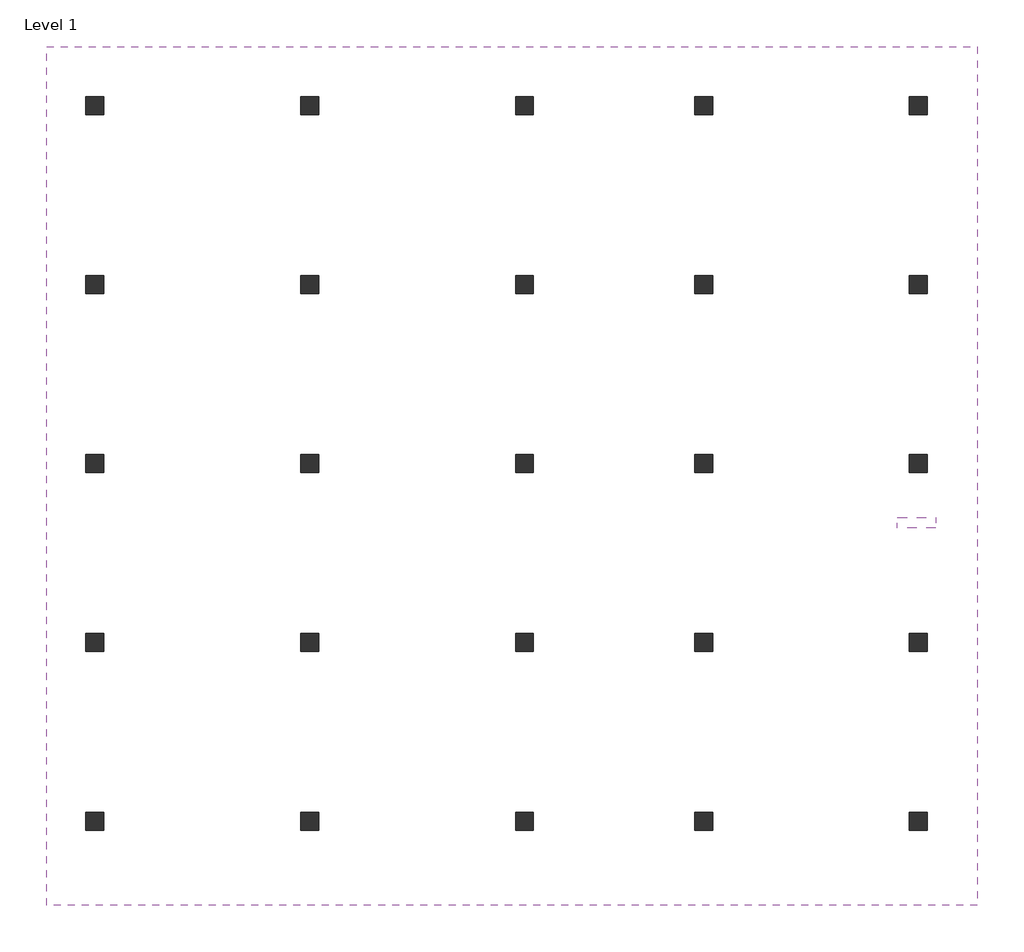
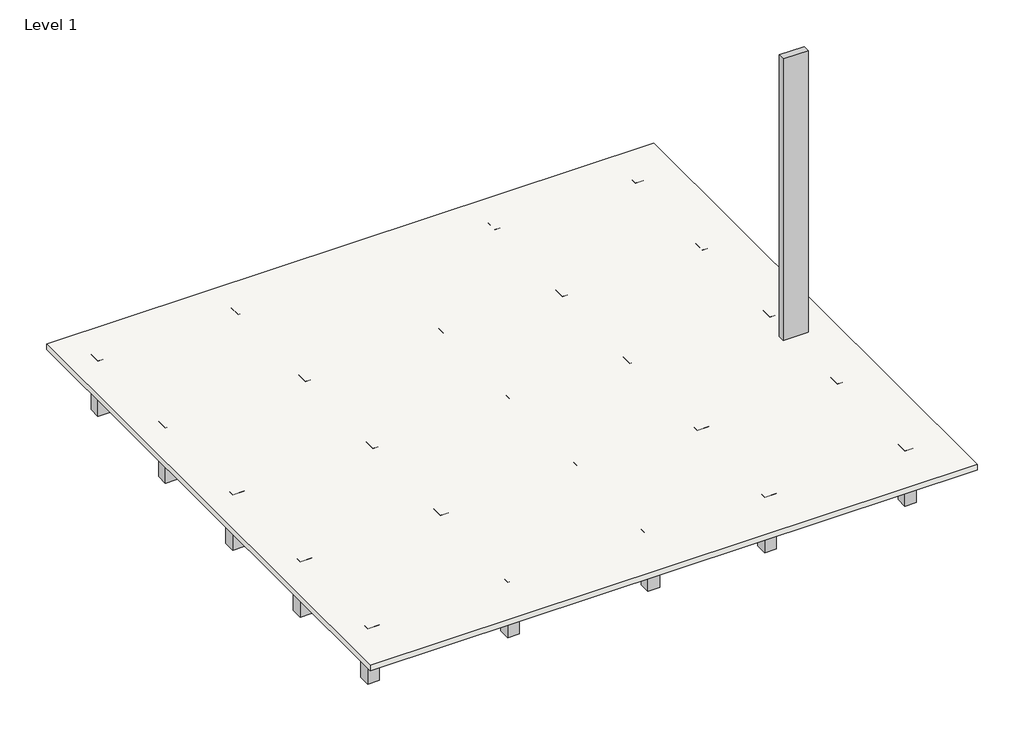
# One storey: 25 columns, 1 proxy, 1 slab.
"""IFC4 building model written with IfcOpenShell, lengths in millimetres."""

from ifc_helpers import new_model, si_unit, frame, origin, place, context, project, spatial, polyline, outline, extrude, transform, mapped, element, save
from components import generic_models_3_generic_models_3_f60183ce, column_c091e905

model = new_model("IFC4")

# Units and contexts
model_context = context("Model", 3, world=origin())
ifc_project = project(units=[si_unit("LENGTHUNIT", "METRE", prefix="MILLI")], contexts=[model_context])

# Site, building, storey
site = spatial("IfcSite", under=ifc_project)
building = spatial("IfcBuilding", under=site)
storey = spatial("IfcBuildingStorey", under=building, Name="Level 1", Elevation=0.0)

# Proxy
placement = place(None, origin())
generic_models_3_generic_models_3_shape = generic_models_3_generic_models_3_f60183ce(model_context)
element("IfcBuildingElementProxy", 1, Name="Generic Models 3 : Generic Models 3", ObjectType="Generic Models 3 : Generic Models 3", at=placement, inside=storey, context=model_context, shape_type="MappedRepresentation", body=[
    mapped(generic_models_3_generic_models_3_shape, transform((0.0, 0.0, 0.0), x_axis=(1.0, 0.0, 0.0), y_axis=(0.0, 1.0, 0.0), z_axis=(0.0, 0.0, 1.0))),
])

# Columns
column_shape = column_c091e905(model_context)
element("IfcColumn", 2, ObjectType="Rectangular Column : 24\" x 24\"", at=placement, inside=storey, context=model_context, shape_type="MappedRepresentation", body=[
    mapped(column_shape, transform((-13731.8638778, 14362.2237525, 0.0), x_axis=(1.0, 0.0, 0.0), y_axis=(0.0, 1.0, 0.0), z_axis=(0.0, 0.0, 1.0))),
])
element("IfcColumn", 3, ObjectType="Rectangular Column : 24\" x 24\"", at=placement, inside=storey, context=model_context, shape_type="MappedRepresentation", body=[
    mapped(column_shape, transform((-6416.6638778, 14362.2237525, 0.0), x_axis=(1.0, 0.0, 0.0), y_axis=(0.0, 1.0, 0.0), z_axis=(0.0, 0.0, 1.0))),
])
element("IfcColumn", 4, ObjectType="Rectangular Column : 24\" x 24\"", at=placement, inside=storey, context=model_context, shape_type="MappedRepresentation", body=[
    mapped(column_shape, transform((898.5361222, 14362.2237525, 0.0), x_axis=(1.0, 0.0, 0.0), y_axis=(0.0, 1.0, 0.0), z_axis=(0.0, 0.0, 1.0))),
])
element("IfcColumn", 5, ObjectType="Rectangular Column : 24\" x 24\"", at=placement, inside=storey, context=model_context, shape_type="MappedRepresentation", body=[
    mapped(column_shape, transform((6994.5361222, 14362.2237525, 0.0), x_axis=(1.0, 0.0, 0.0), y_axis=(0.0, 1.0, 0.0), z_axis=(0.0, 0.0, 1.0))),
])
element("IfcColumn", 6, ObjectType="Rectangular Column : 24\" x 24\"", at=placement, inside=storey, context=model_context, shape_type="MappedRepresentation", body=[
    mapped(column_shape, transform((14309.7361222, 14362.2237525, 0.0), x_axis=(1.0, 0.0, 0.0), y_axis=(0.0, 1.0, 0.0), z_axis=(0.0, 0.0, 1.0))),
])
element("IfcColumn", 7, ObjectType="Rectangular Column : 24\" x 24\"", at=placement, inside=storey, context=model_context, shape_type="MappedRepresentation", body=[
    mapped(column_shape, transform((14309.7361222, 8266.2237525, 0.0), x_axis=(1.0, 0.0, 0.0), y_axis=(0.0, 1.0, 0.0), z_axis=(0.0, 0.0, 1.0))),
])
element("IfcColumn", 8, ObjectType="Rectangular Column : 24\" x 24\"", at=placement, inside=storey, context=model_context, shape_type="MappedRepresentation", body=[
    mapped(column_shape, transform((6994.5361222, 8266.2237525, 0.0), x_axis=(1.0, 0.0, 0.0), y_axis=(0.0, 1.0, 0.0), z_axis=(0.0, 0.0, 1.0))),
])
element("IfcColumn", 9, ObjectType="Rectangular Column : 24\" x 24\"", at=placement, inside=storey, context=model_context, shape_type="MappedRepresentation", body=[
    mapped(column_shape, transform((898.5361222, 8266.2237525, 0.0), x_axis=(1.0, 0.0, 0.0), y_axis=(0.0, 1.0, 0.0), z_axis=(0.0, 0.0, 1.0))),
])
element("IfcColumn", 10, ObjectType="Rectangular Column : 24\" x 24\"", at=placement, inside=storey, context=model_context, shape_type="MappedRepresentation", body=[
    mapped(column_shape, transform((-6416.6638778, 8266.2237525, 0.0), x_axis=(1.0, 0.0, 0.0), y_axis=(0.0, 1.0, 0.0), z_axis=(0.0, 0.0, 1.0))),
])
element("IfcColumn", 11, ObjectType="Rectangular Column : 24\" x 24\"", at=placement, inside=storey, context=model_context, shape_type="MappedRepresentation", body=[
    mapped(column_shape, transform((-13731.8638778, 8266.2237525, 0.0), x_axis=(1.0, 0.0, 0.0), y_axis=(0.0, 1.0, 0.0), z_axis=(0.0, 0.0, 1.0))),
])
element("IfcColumn", 12, ObjectType="Rectangular Column : 24\" x 24\"", at=placement, inside=storey, context=model_context, shape_type="MappedRepresentation", body=[
    mapped(column_shape, transform((-13731.8638778, 2170.2237525, 0.0), x_axis=(1.0, 0.0, 0.0), y_axis=(0.0, 1.0, 0.0), z_axis=(0.0, 0.0, 1.0))),
])
element("IfcColumn", 13, ObjectType="Rectangular Column : 24\" x 24\"", at=placement, inside=storey, context=model_context, shape_type="MappedRepresentation", body=[
    mapped(column_shape, transform((-6416.6638778, 2170.2237525, 0.0), x_axis=(1.0, 0.0, 0.0), y_axis=(0.0, 1.0, 0.0), z_axis=(0.0, 0.0, 1.0))),
])
element("IfcColumn", 14, ObjectType="Rectangular Column : 24\" x 24\"", at=placement, inside=storey, context=model_context, shape_type="MappedRepresentation", body=[
    mapped(column_shape, transform((898.5361222, 2170.2237525, 0.0), x_axis=(1.0, 0.0, 0.0), y_axis=(0.0, 1.0, 0.0), z_axis=(0.0, 0.0, 1.0))),
])
element("IfcColumn", 15, ObjectType="Rectangular Column : 24\" x 24\"", at=placement, inside=storey, context=model_context, shape_type="MappedRepresentation", body=[
    mapped(column_shape, transform((6994.5361222, 2170.2237525, 0.0), x_axis=(1.0, 0.0, 0.0), y_axis=(0.0, 1.0, 0.0), z_axis=(0.0, 0.0, 1.0))),
])
element("IfcColumn", 16, ObjectType="Rectangular Column : 24\" x 24\"", at=placement, inside=storey, context=model_context, shape_type="MappedRepresentation", body=[
    mapped(column_shape, transform((14309.7361222, 2170.2237525, 0.0), x_axis=(1.0, 0.0, 0.0), y_axis=(0.0, 1.0, 0.0), z_axis=(0.0, 0.0, 1.0))),
])
element("IfcColumn", 17, ObjectType="Rectangular Column : 24\" x 24\"", at=placement, inside=storey, context=model_context, shape_type="MappedRepresentation", body=[
    mapped(column_shape, transform((14309.7361222, -3925.7762475, 0.0), x_axis=(1.0, 0.0, 0.0), y_axis=(0.0, 1.0, 0.0), z_axis=(0.0, 0.0, 1.0))),
])
element("IfcColumn", 18, ObjectType="Rectangular Column : 24\" x 24\"", at=placement, inside=storey, context=model_context, shape_type="MappedRepresentation", body=[
    mapped(column_shape, transform((6994.5361222, -3925.7762475, 0.0), x_axis=(1.0, 0.0, 0.0), y_axis=(0.0, 1.0, 0.0), z_axis=(0.0, 0.0, 1.0))),
])
element("IfcColumn", 19, ObjectType="Rectangular Column : 24\" x 24\"", at=placement, inside=storey, context=model_context, shape_type="MappedRepresentation", body=[
    mapped(column_shape, transform((898.5361222, -3925.7762475, 0.0), x_axis=(1.0, 0.0, 0.0), y_axis=(0.0, 1.0, 0.0), z_axis=(0.0, 0.0, 1.0))),
])
element("IfcColumn", 20, ObjectType="Rectangular Column : 24\" x 24\"", at=placement, inside=storey, context=model_context, shape_type="MappedRepresentation", body=[
    mapped(column_shape, transform((-6416.6638778, -3925.7762475, 0.0), x_axis=(1.0, 0.0, 0.0), y_axis=(0.0, 1.0, 0.0), z_axis=(0.0, 0.0, 1.0))),
])
element("IfcColumn", 21, ObjectType="Rectangular Column : 24\" x 24\"", at=placement, inside=storey, context=model_context, shape_type="MappedRepresentation", body=[
    mapped(column_shape, transform((-13731.8638778, -3925.7762475, 0.0), x_axis=(1.0, 0.0, 0.0), y_axis=(0.0, 1.0, 0.0), z_axis=(0.0, 0.0, 1.0))),
])
element("IfcColumn", 22, ObjectType="Rectangular Column : 24\" x 24\"", at=placement, inside=storey, context=model_context, shape_type="MappedRepresentation", body=[
    mapped(column_shape, transform((-13731.8638778, -10021.7762475, 0.0), x_axis=(1.0, 0.0, 0.0), y_axis=(0.0, 1.0, 0.0), z_axis=(0.0, 0.0, 1.0))),
])
element("IfcColumn", 23, ObjectType="Rectangular Column : 24\" x 24\"", at=placement, inside=storey, context=model_context, shape_type="MappedRepresentation", body=[
    mapped(column_shape, transform((-6416.6638778, -10021.7762475, 0.0), x_axis=(1.0, 0.0, 0.0), y_axis=(0.0, 1.0, 0.0), z_axis=(0.0, 0.0, 1.0))),
])
element("IfcColumn", 24, ObjectType="Rectangular Column : 24\" x 24\"", at=placement, inside=storey, context=model_context, shape_type="MappedRepresentation", body=[
    mapped(column_shape, transform((898.5361222, -10021.7762475, 0.0), x_axis=(1.0, 0.0, 0.0), y_axis=(0.0, 1.0, 0.0), z_axis=(0.0, 0.0, 1.0))),
])
element("IfcColumn", 25, ObjectType="Rectangular Column : 24\" x 24\"", at=placement, inside=storey, context=model_context, shape_type="MappedRepresentation", body=[
    mapped(column_shape, transform((6994.5361222, -10021.7762475, 0.0), x_axis=(1.0, 0.0, 0.0), y_axis=(0.0, 1.0, 0.0), z_axis=(0.0, 0.0, 1.0))),
])
element("IfcColumn", 26, ObjectType="Rectangular Column : 24\" x 24\"", at=placement, inside=storey, context=model_context, shape_type="MappedRepresentation", body=[
    mapped(column_shape, transform((14309.7361222, -10021.7762475, 0.0), x_axis=(1.0, 0.0, 0.0), y_axis=(0.0, 1.0, 0.0), z_axis=(0.0, 0.0, 1.0))),
])

# Slab
element("IfcSlab", 27, at=placement, inside=storey, context=model_context, shape_type="SweptSolid", body=[
    extrude(outline(polyline([(16321.4289933, 16374.4250499), (16321.4289933, -12886.3749501), (-15377.7710067, -12886.3749501), (-15377.7710067, 16374.4250499), (16321.4289933, 16374.4250499)])), frame((0.0, 0.0, 2743.2), z_axis=(0.0, 0.0, 1.0), x_axis=(1.0, 0.0, 0.0)), (0.0, 0.0, 1.0), 304.8),
])

save(model, "model.ifc")

# Revit data of these elements
# Grids (mm)
#   "1": line (-13731.864, -18407.69) -> (-13731.864, 14362.224)
#   "2": line (22325.703, 14362.224) -> (-13731.864, 14362.224)
#   "3": line (22325.703, 8266.224) -> (-13731.864, 8266.224)
#   "4": line (22325.703, 2170.224) -> (-13731.864, 2170.224)
#   "5": line (22325.703, -3925.776) -> (-13731.864, -3925.776)
#   "6": line (22325.703, -10021.776) -> (-13731.864, -10021.776)
#   "7": line (22325.703, -18407.69) -> (-13731.864, -18407.69)
#   "8": line (-6416.664, -18407.69) -> (-6416.664, 14362.224)
#   "9": line (898.536, -18407.69) -> (898.536, 14362.224)
#   "10": line (6994.536, -18407.69) -> (6994.536, 14362.224)
#   "11": line (14309.736, -18407.69) -> (14309.736, 14362.224)
# Type "Rectangular Column : 24\" x 24\""
#   Assembly Code = "B1010200"
#   Depth = 2' - 0"
#   Offset Base = 0' - 0"
#   Offset Top = 0' - 0"
#   Width = 2' - 0"
#   Material = none
# Type
#   Assembly Code = "B1010"
#   Function = 0
#   Layers, outside or top first: 1' - 0" "Tile, Porcelain, 4in" (function 1)
# Element 1 (IfcBuildingElementProxy, "Generic Models 3 : Generic Models 3")
#   Phase Created = New Construction
# Elements 2, 3, 4, 5, 6, 7, 8, 9, 10, 11, 12, 13, 14, 15, 16, 17, 18, 19, 20, 21, 22, 23, 24, 25, 26 (IfcColumn, "Rectangular Column : 24\" x 24\"")
#   Phase Created = New Construction
# Element 27 (IfcSlab)
#   Height Offset From Level = 10' - 0"
#   Phase Created = New Construction
#   Materials on its faces: "Tile, Porcelain, 4in"
# Materials
#   "Tile, Porcelain, 4in": class "Generic", colour RGB 89 87 158, transparency 0, Description = "Porcelain tile, 4\", white", Cost = 0
